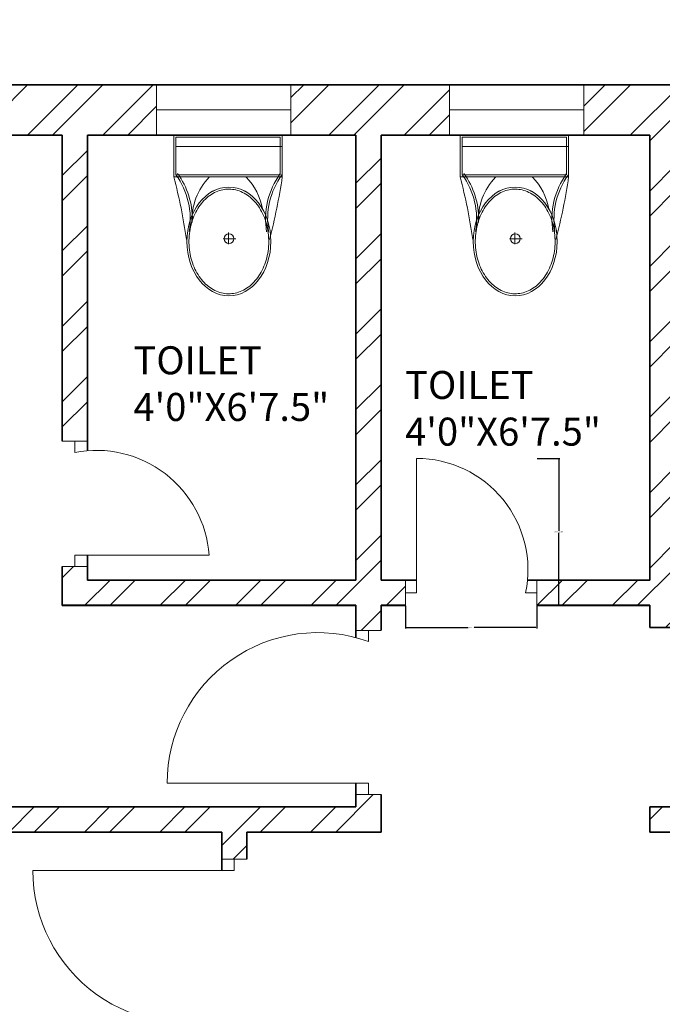
# Model space of a CAD drawing. Units: inches. Extents: x 2120 to 4013, y 1390 to 3019.
# Tile 33 of 59: x 2356 to 2470, y 2188 to 2364. Entities that reach past the tile are written whole.
import ezdxf

# ---------------------------------------------------------------- set-up
doc = ezdxf.new("R2010")
doc.units = ezdxf.units.IN
for name, color, linetype, lineweight in [('A-ANNO-DIMS', 2, 'Continuous', 18), ('A-AREA-IDEN', 7, 'Continuous', 18), ('A-DOOR', 3, 'Continuous', 18), ('A-FLOR-FIXT', 9, 'Continuous', 18), ('A-GLAZ', 4, 'Continuous', 18), ('A-WALL', 7, 'Continuous', 35), ('A-WALL-PATT', 252, 'Continuous', 13)]:
    doc.layers.add(name, color=color, linetype=linetype, lineweight=lineweight)
doc.styles.get("Standard").update_dxf_attribs({"font": 'arial.ttf'})
doc.dimstyles.get("Standard").update_dxf_attribs({"dimtxt": 0.18, "dimasz": 0.18, "dimexe": 0.18, "dimexo": 0.0625, "dimgap": 0.09, "dimtad": 0, "dimtih": 1, "dimtoh": 1, "dimdec": 4, "dimzin": 0, "dimdsep": 46, "dimtxsty": 'Standard', "dimcen": 0.09, "dimadec": 0, "dimazin": 0, "dimtfac": 1, "dimtdec": 4, "dimtofl": 0, "dimtmove": 0, "dimatfit": 3, "dimfxl": 1, "dimtolj": 1, "dimtzin": 0, "dimarcsym": 0})

# ---------------------------------------------------------------- blocks, each defined once
blk = doc.blocks.new('A$C31115884')
for p, q in [((257.5, 466.4), (257.5, 523.2)), ((283.1, 497.7), (223.4, 497.7)), ((0, 200), (0, 0)), ((520, 200), (0, 200)), ((10, 190), (10, 10)), ((510, 190), (10, 190)), ((510, 10), (510, 190)), ((520, 0), (520, 200)), ((510, 54.5), (0, 54.5)), ((10, 10), (510, 10)), ((0, 0), (520, 0))]:
    blk.add_line(p, q)
blk.add_circle((255.6, 496.4), 23.6)
for centre, radius, start, end in [((2777.7, -204.6), 2807, 165.4549, 171.7133), ((3237, 905), 2807, 188.2867, 194.5451), ((-294.5, 403.3), 364.7, 324.2091, 9.3499), ((-294.5, 403.3), 374.7, 324.2091, 9.3499), ((805.8, 403.3), 364.7, 170.6501, 215.7909), ((139.5, 406.2), 293.5, 315.8436, 2.6563), ((805.8, 403.3), 374.7, 179.2036, 215.7909), ((383.6, 406.2), 293.5, 190.2774, 224.1564)]:
    blk.add_arc(centre, radius, start, end)
blk.add_ellipse((256.2, 509.9), major_axis=(0, -260.7), ratio=0.772727)
blk.add_open_spline([(256.2, 259.2), (263.1, 259.2), (270, 259.7), (287.8, 262.3), (298.7, 265.1), (319.9, 273.1), (330.2, 278.4), (350.1, 291.1), (359.7, 298.7), (377.7, 315.9), (386.2, 325.5), (401.7, 346.6), (408.8, 358.1), (421.3, 382.5), (426.8, 395.5), (435.9, 422.4), (439.5, 436.4), (444.8, 465.1), (446.5, 479.7), (447.9, 509.2), (447.6, 524), (445, 553.3), (442.7, 567.8), (436.3, 596), (432.1, 609.7), (421.9, 636), (416, 648.6), (402.5, 672.1), (395, 683), (378.6, 703), (369.8, 712.1), (351.1, 728), (341.3, 734.8), (320.9, 746.2), (310.4, 750.7), (288.9, 757.3), (278, 759.4), (256, 761), (245, 760.6), (223.1, 757.2), (212.3, 754.3), (191.1, 746.1), (180.8, 740.7), (160.9, 727.8), (151.4, 720.1), (133.5, 702.7), (125.1, 693), (109.6, 671.7), (102.6, 660.2), (90.2, 635.7), (84.9, 622.7), (76, 595.6), (72.4, 581.6), (67.2, 552.9), (65.6, 538.2), (64.4, 508.8), (64.8, 494), (67.5, 464.7), (69.9, 450.2), (76.6, 422), (80.8, 408.3), (91.1, 382.2), (97.2, 369.7), (110.8, 346.3), (118.4, 335.4), (134.8, 315.6), (143.7, 306.7), (162.4, 290.9), (172.3, 284.2), (192.8, 273), (203.3, 268.6), (224.8, 262.2), (235.8, 260.2), (249.9, 259.3), (253, 259.2), (256.2, 259.2)], degree=3, knots=[0, 0, 0, 0, 0.110105, 0.110105, 0.285049, 0.285049, 0.459994, 0.459994, 0.634938, 0.634938, 0.809882, 0.809882, 0.984827, 0.984827, 1.159771, 1.159771, 1.334715, 1.334715, 1.50966, 1.50966, 1.684604, 1.684604, 1.859549, 1.859549, 2.034493, 2.034493, 2.209437, 2.209437, 2.384382, 2.384382, 2.559326, 2.559326, 2.73427, 2.73427, 2.909215, 2.909215, 3.084159, 3.084159, 3.259103, 3.259103, 3.434048, 3.434048, 3.608992, 3.608992, 3.783936, 3.783936, 3.958881, 3.958881, 4.133825, 4.133825, 4.30877, 4.30877, 4.483714, 4.483714, 4.658658, 4.658658, 4.833603, 4.833603, 5.008547, 5.008547, 5.183491, 5.183491, 5.358436, 5.358436, 5.53338, 5.53338, 5.708324, 5.708324, 5.883269, 5.883269, 6.058213, 6.058213, 6.233158, 6.233158, 6.283185, 6.283185, 6.283185, 6.283185])
blk = doc.blocks.new('DOOR-SWING-24IN-96p73DEG')
for p, q in [((4.5, 22.36), (0, 22.36)), ((0, 22.36), (2.25, 22.36)), ((2.25, 22.36), (2.25, 20.36)), ((2.25, 0), (2.25, 2)), ((2.25, 2), (26.25, 2)), ((4.5, 0), (0, 0)), ((0, 0), (2.25, 0))]:
    blk.add_line(p, q)
blk.add_arc((6.09, 0.51), 20.22, 4.2154, 100.9483)
blk = doc.blocks.new('DOOR-SWING-24IN-101p88DEG')
for p, q in [((2, 2.25), (2, 26.25)), ((0, 4.5), (0, 0)), ((23.48, 4.5), (23.48, 0)), ((0, 0), (0, 2.25)), ((0, 2.25), (2, 2.25)), ((23.48, 2.25), (21.48, 2.25)), ((23.48, 0), (23.48, 2.25))]:
    blk.add_line(p, q)
blk.add_arc((2, 6.35), 19.9, 348.1217, 90)
blk = doc.blocks.new('DOOR-SWING-36IN-109p78DEG')
for p, q in [((33.75, 29.31), (38.25, 29.31)), ((38.25, 29.31), (36, 29.31)), ((36, 29.31), (36, 27.31)), ((36, 2), (0, 2)), ((36, 0), (36, 2)), ((33.75, 0), (38.25, 0)), ((38.25, 0), (35.24, 0)), ((35.24, 0), (36, 0))]:
    blk.add_line(p, q)
blk.add_arc((26.9, 2), 26.9, 70.2228, 180)
blk = doc.blocks.new('DOOR-SWING-36IN-108p68DEG')
for p, q in [((38.25, 29.83), (33.75, 29.83)), ((33.75, 29.83), (36, 29.83)), ((36, 29.83), (36, 27.83)), ((36, 27.83), (0, 27.83)), ((36, 0), (36, 2)), ((33.75, 0), (38.25, 0)), ((38.25, 0), (36, 0))]:
    blk.add_line(p, q)
blk.add_arc((27.27, 27.83), 27.27, 180, 288.6764)
blk = doc.blocks.new('WIN-PLAN-24IN')
for p, q in [((0, 0), (0, 9)), ((0, 9), (0, 4.5)), ((24, 4.5), (24, 9)), ((24, 9), (24, 0)), ((0, 4.5), (24, 4.5)), ((0, 0), (0, 0))]:
    blk.add_line(p, q)
blk = doc.blocks.new('WIN-PLAN-24IN-02')
for p, q in [((0, 0), (0, 9)), ((0, 9), (0, 4.5)), ((24, 4.5), (24, 9)), ((24, 9), (24, 0)), ((0, 4.5), (24, 4.5))]:
    blk.add_line(p, q)
blk = doc.blocks.new('*D115')
at = {"layer": 'A-ANNO-DIMS', "color": 0, "lineweight": -2, "transparency": 16777216}
for p, q in [((2448.11, 2285.78), (2452.17, 2285.78)), ((2451.99, 2285.6), (2451.99, 2272.84)), ((2451.99, 2259.71), (2451.99, 2272.47)), ((2448.11, 2259.53), (2452.17, 2259.53))]:
    blk.add_line(p, q, dxfattribs=at)
at = {"layer": 'A-ANNO-DIMS', "color": 0, "transparency": 16777216}
for points in [[(2451.96, 2285.6), (2452.02, 2285.6), (2451.99, 2285.78)], [(2451.96, 2259.71), (2452.02, 2259.71), (2451.99, 2259.53)]]:
    blk.add_solid(points, dxfattribs=at)
at = {"layer": 'Defpoints', "color": 0, "transparency": 16777216}
for p in [(2448.05, 2285.78), (2451.99, 2285.78), (2448.05, 2259.53)]:
    blk.add_point(p, dxfattribs=at)
at = {"layer": 'A-ANNO-DIMS', "color": 0, "transparency": 16777216, "insert": (2451.99, 2272.66), "char_height": 0.18, "attachment_point": 5}
blk.add_mtext('\\A1;SWING 26 TYP.', dxfattribs=at)
blk = doc.blocks.new('*D116')
at = {"layer": 'A-ANNO-DIMS', "color": 0, "lineweight": -2, "transparency": 16777216}
for p, q in [((2424.57, 2259.47), (2424.57, 2255.41)), ((2448.05, 2259.47), (2448.05, 2255.41)), ((2424.75, 2255.59), (2435.78, 2255.59)), ((2447.87, 2255.59), (2436.84, 2255.59))]:
    blk.add_line(p, q, dxfattribs=at)
at = {"layer": 'A-ANNO-DIMS', "color": 0, "transparency": 16777216}
for points in [[(2424.75, 2255.62), (2424.75, 2255.56), (2424.57, 2255.59)], [(2447.87, 2255.62), (2447.87, 2255.56), (2448.05, 2255.59)]]:
    blk.add_solid(points, dxfattribs=at)
at = {"layer": 'Defpoints', "color": 0, "transparency": 16777216}
for p in [(2424.57, 2259.53), (2448.05, 2259.53), (2448.05, 2255.59)]:
    blk.add_point(p, dxfattribs=at)
at = {"layer": 'A-ANNO-DIMS', "color": 0, "transparency": 16777216, "insert": (2436.31, 2255.59), "char_height": 0.18, "attachment_point": 5}
blk.add_mtext('\\A1;23 TYP.', dxfattribs=at)
blk = doc.blocks.new('*D211')
at = {"layer": 'A-ANNO-DIMS', "color": 0, "lineweight": -2, "transparency": 16777216}
for p, q in [((2262.73, 2352.59), (2262.73, 2397.71)), ((2262.91, 2397.53), (2635.95, 2397.53)), ((3009.55, 2397.53), (2636.52, 2397.53)), ((3009.73, 2352.59), (3009.73, 2397.71))]:
    blk.add_line(p, q, dxfattribs=at)
at = {"layer": 'A-ANNO-DIMS', "color": 0, "transparency": 16777216}
for points in [[(2262.91, 2397.56), (2262.91, 2397.5), (2262.73, 2397.53)], [(3009.55, 2397.56), (3009.55, 2397.5), (3009.73, 2397.53)]]:
    blk.add_solid(points, dxfattribs=at)
at = {"layer": 'Defpoints', "color": 0, "transparency": 16777216}
for p in [(3009.73, 2397.53), (2262.73, 2352.53), (3009.73, 2352.53)]:
    blk.add_point(p, dxfattribs=at)
at = {"layer": 'A-ANNO-DIMS', "color": 0, "transparency": 16777216, "insert": (2636.23, 2397.53), "char_height": 0.18, "attachment_point": 5}
blk.add_mtext('\\A1;747', dxfattribs=at)

msp = doc.modelspace()

# ---------------------------------------------------------------- hatches: boundary and pattern name
at = {"layer": 'A-WALL-PATT'}
h = msp.add_hatch(dxfattribs=at)
h.set_pattern_fill('ANSI32', color=256)
h.paths.add_polyline_path([(2271.7331, 2343.531), (2283.3788, 2343.531), (2283.3788, 2348.031), (2283.3788, 2352.5306), (2262.7331, 2352.5306), (2262.7331, 2182.638), (2267.2331, 2182.638), (2271.7331, 2182.638), (2271.7331, 2219.031), (2391.7331, 2219.031), (2391.7331, 2214.189), (2393.9831, 2214.189), (2396.2331, 2214.189), (2396.2331, 2219.031), (2420.2331, 2219.031), (2420.2331, 2225.7535), (2417.2197, 2225.7535), (2415.7331, 2225.7535), (2415.7331, 2223.5306), (2271.7331, 2223.5306)])
h.paths.add_polyline_path([(2380.0942, 2352.5306), (2343.3788, 2352.5306), (2343.3788, 2343.531), (2363.2331, 2343.531), (2363.2331, 2288.8489), (2365.4831, 2288.8489), (2367.7331, 2288.8489), (2367.7331, 2343.531), (2380.0942, 2343.531)], flags=17)
h.paths.add_polyline_path([(2432.4339, 2352.5306), (2404.0943, 2352.5306), (2404.0943, 2343.531), (2415.7331, 2343.531), (2415.7331, 2264.0306), (2367.7331, 2264.0306), (2367.7331, 2266.4872), (2363.2331, 2266.4872), (2363.2331, 2259.531), (2367.7331, 2259.531), (2415.7331, 2259.531), (2415.7331, 2255.0658), (2420.2331, 2255.0658), (2420.2331, 2259.531), (2424.5717, 2259.531), (2424.5717, 2261.781), (2424.5717, 2264.0306), (2420.2331, 2264.0306), (2420.2331, 2343.531), (2432.4339, 2343.531)])
h.paths.add_polyline_path([(2508.9115, 2352.5306), (2456.4339, 2352.5306), (2456.4339, 2343.531), (2468.2331, 2343.531), (2468.2331, 2264.0306), (2448.0487, 2264.0306), (2448.0487, 2259.531), (2468.2331, 2259.531), (2468.2331, 2255.5496), (2472.7331, 2255.5496), (2472.7331, 2343.531), (2508.9115, 2343.531)])
h.paths.add_polyline_path([(2637.7331, 2352.5306), (2544.9116, 2352.5306), (2544.9116, 2343.531), (2589.7331, 2343.531), (2633.2331, 2343.531), (2637.7331, 2343.531)])
h.paths.add_polyline_path([(2594.2331, 2343.5306), (2589.7331, 2343.5306), (2589.7331, 2259.5306), (2589.7331, 2252.4915), (2591.9831, 2252.4915), (2594.2331, 2252.4915)])
h.paths.add_polyline_path([(2637.7331, 2223.5306), (2594.2331, 2223.5306), (2594.2331, 2230.1988), (2591.9831, 2230.1988), (2589.7331, 2230.1988), (2589.7331, 2223.5306), (2472.7331, 2223.5306), (2468.2331, 2223.5306), (2468.2331, 2219.031), (2628.7331, 2219.031), (2628.7331, 2138.031), (2637.7331, 2138.031)])
h.paths.add_polyline_path([(3822.6535, 2458.4402), (3874.9468, 2458.4402), (3874.9468, 2476.9866), (3822.6535, 2476.9866)], flags=9)
h.paths.add_polyline_path([(3834.6921, 2781.8174), (3935.9206, 2781.8174), (3935.9206, 2800.3638), (3834.6921, 2800.3638)], flags=9)
h.paths.add_polyline_path([(3832.2843, 2837.9683), (3884.5776, 2837.9683), (3884.5776, 2856.5146), (3832.2843, 2856.5146)], flags=9)
h.paths.add_polyline_path([(3830.9388, 2861.4782), (3956.8958, 2861.4782), (3956.8958, 2880.0245), (3830.9388, 2880.0245)], flags=9)
h.paths.add_polyline_path([(3870.6966, 2352.5752), (3887.9272, 2352.5752), (3887.9272, 2377.3037), (3870.6966, 2377.3037)], flags=9)
h.paths.add_polyline_path([(3289.2701, 2413.161), (3435.2223, 2413.161), (3435.2223, 2450.2538), (3289.2701, 2450.2538)], flags=9)
h.paths.add_polyline_path([(2487.6944, 2414.3601), (2637.8335, 2414.3601), (2637.8335, 2451.4528), (2487.6944, 2451.4528)], flags=9)
h.paths.add_polyline_path([(2567.3724, 1457.9199), (2815.296, 1457.9199), (2815.296, 1495.0127), (2567.3724, 1495.0127)], flags=9)
h.paths.add_polyline_path([(2655.3825, 2093.2363), (2685.9555, 2093.2363), (2685.9555, 2111.8937), (2655.3825, 2111.8937)], flags=9)
h.paths.add_polyline_path([(2543.9218, 1550.6671), (2587.8406, 1550.6671), (2587.8406, 1569.3244), (2543.9218, 1569.3244)], flags=9)
h.paths.add_polyline_path([(2905.1384, 1543.8113), (2949.0572, 1543.8113), (2949.0572, 1562.4686), (2905.1384, 1562.4686)], flags=9)
h.paths.add_polyline_path([(2736.4118, 1702.4736), (2784.2153, 1702.4736), (2784.2153, 1721.1309), (2736.4118, 1721.1309)], flags=9)
h.paths.add_polyline_path([(2912.8666, 1710.4168), (2951.707, 1710.4168), (2951.707, 1729.0741), (2912.8666, 1729.0741)], flags=9)
h.paths.add_polyline_path([(2923.5785, 1763.5038), (2959.7279, 1763.5038), (2959.7279, 1782.1611), (2923.5785, 1782.1611)], flags=9)
h.paths.add_polyline_path([(2925.2114, 1809.6137), (2967.1861, 1809.6137), (2967.1861, 1828.271), (2925.2114, 1828.271)], flags=9)
h.paths.add_polyline_path([(2996.2711, 1878.9003), (2996.2711, 1913.109), (2977.6138, 1913.109), (2977.6138, 1878.9003)], flags=9)
h.paths.add_polyline_path([(2883.0859, 1895.7192), (2927.1855, 1895.7192), (2927.1855, 1914.3766), (2883.0859, 1914.3766)], flags=9)
h.paths.add_polyline_path([(2787.3924, 1810.8013), (2841.0213, 1810.8013), (2841.0213, 1829.4587), (2787.3924, 1829.4587)], flags=9)
h.paths.add_polyline_path([(2775.6399, 2101.7395), (2829.2689, 2101.7395), (2829.2689, 2120.3968), (2775.6399, 2120.3968)], flags=9)
h.paths.add_polyline_path([(2913.0263, 2075.817), (2951.8667, 2075.817), (2951.8667, 2094.4744), (2913.0263, 2094.4744)], flags=9)
h.paths.add_polyline_path([(2929.966, 2133.3669), (2966.1154, 2133.3669), (2966.1154, 2152.0243), (2929.966, 2152.0243)], flags=9)
h.paths.add_polyline_path([(2932.7502, 2182.6088), (2968.8996, 2182.6088), (2968.8996, 2201.2662), (2932.7502, 2201.2662)], flags=9)
h.paths.add_polyline_path([(2996.0681, 2266.3173), (2996.0681, 2300.5261), (2977.4108, 2300.5261), (2977.4108, 2266.3173)], flags=9)
h.paths.add_polyline_path([(2885.1039, 2279.2186), (2929.2035, 2279.2186), (2929.2035, 2297.8759), (2885.1039, 2297.8759)], flags=9)
h.paths.add_polyline_path([(2735.7042, 2218.3197), (2783.5078, 2218.3197), (2783.5078, 2236.9771), (2735.7042, 2236.9771)], flags=9)
h.paths.add_polyline_path([(2635.6049, 2044.0085), (2648.9678, 2044.0085), (2648.9678, 2054.312), (2635.6049, 2054.312)], flags=9)
h.paths.add_polyline_path([(2714.0148, 1923.0473), (2727.3777, 1923.0473), (2727.3777, 1933.3508), (2714.0148, 1933.3508)], flags=9)
h.paths.add_polyline_path([(2709.0345, 1988.1628), (2722.3974, 1988.1628), (2722.3974, 1998.4663), (2709.0345, 1998.4663)], flags=9)
h.paths.add_polyline_path([(2592.8935, 1962.1763), (2606.2564, 1962.1763), (2606.2564, 1972.4799), (2592.8935, 1972.4799)], flags=9)
h.paths.add_polyline_path([(2618.3996, 1985.9724), (2644.1942, 1985.9724), (2644.1942, 1996.2759), (2618.3996, 1996.2759)], flags=9)
h.paths.add_polyline_path([(2601.279, 1920.5869), (2614.6419, 1920.5869), (2614.6419, 1930.8904), (2601.279, 1930.8904)], flags=9)
h.paths.add_polyline_path([(2692.3278, 1932.7645), (2704.5311, 1932.7645), (2704.5311, 1943.0681), (2692.3278, 1943.0681)], flags=9)
h.paths.add_polyline_path([(2311.122, 1672.7318), (2355.0408, 1672.7318), (2355.0408, 1691.3892), (2311.122, 1691.3892)], flags=9)
h.paths.add_polyline_path([(2456.2551, 1632.3198), (2492.4796, 1632.3198), (2492.4796, 1650.9772), (2456.2551, 1650.9772)], flags=9)
h.paths.add_polyline_path([(2401.0766, 1631.4793), (2437.301, 1631.4793), (2437.301, 1650.1367), (2401.0766, 1650.1367)], flags=9)
h.paths.add_polyline_path([(2546.7054, 1700.9235), (2594.509, 1700.9235), (2594.509, 1719.5809), (2546.7054, 1719.5809)], flags=9)
h.paths.add_polyline_path([(2445.4866, 1766.9937), (2497.5261, 1766.9937), (2497.5261, 1785.651), (2445.4866, 1785.651)], flags=9)
h.paths.add_polyline_path([(2287.9992, 1739.7675), (2326.8396, 1739.7675), (2326.8396, 1758.4248), (2287.9992, 1758.4248)], flags=9)
h.paths.add_polyline_path([(2458.5279, 1924.7607), (2510.5675, 1924.7607), (2510.5675, 1943.4181), (2458.5279, 1943.4181)], flags=9)
h.paths.add_polyline_path([(2309.2811, 1902.7642), (2345.4305, 1902.7642), (2345.4305, 1921.4215), (2309.2811, 1921.4215)], flags=9)
h.paths.add_polyline_path([(2490.7554, 2018.9392), (2530.7896, 2018.9392), (2530.7896, 2037.5965), (2490.7554, 2037.5965)], flags=9)
h.paths.add_polyline_path([(2402.143, 2024.7393), (2438.5414, 2024.7393), (2438.5414, 2043.3966), (2402.143, 2043.3966)], flags=9)
h.paths.add_polyline_path([(2287.856, 1931.7926), (2326.6964, 1931.7926), (2326.6964, 1950.4499), (2287.856, 1950.4499)], flags=9)
h.paths.add_polyline_path([(2281.7979, 2193.5771), (2320.6383, 2193.5771), (2320.6383, 2212.2344), (2281.7979, 2212.2344)], flags=25)
h.paths.add_polyline_path([(2484.0754, 2093.892), (2536.115, 2093.892), (2536.115, 2112.5494), (2484.0754, 2112.5494)], flags=9)
h.paths.add_polyline_path([(2624.7948, 2281.8639), (2624.7948, 2311.4137), (2606.1375, 2311.4137), (2606.1375, 2281.8639)], flags=9)
h.paths.add_polyline_path([(2507.5036, 2290.3639), (2541.934, 2290.3639), (2541.934, 2309.0212), (2507.5036, 2309.0212)], flags=9)
h.paths.add_polyline_path([(2423.1076, 2285.2202), (2459.332, 2285.2202), (2459.332, 2303.8776), (2423.1076, 2303.8776)], flags=9)
h.paths.add_polyline_path([(2374.5467, 2289.6272), (2410.7711, 2289.6272), (2410.7711, 2308.2846), (2374.5467, 2308.2846)], flags=25)
h.paths.add_polyline_path([(2277.4907, 2227.5651), (2316.3311, 2227.5651), (2316.3311, 2246.2224), (2277.4907, 2246.2224)], flags=25)
h.paths.add_polyline_path([(2655.3825, 2093.2367), (2685.9555, 2093.2367), (2685.9555, 2111.894), (2655.3825, 2111.894)], flags=9)
h.paths.add_polyline_path([(2543.9217, 1550.6674), (2587.8406, 1550.6674), (2587.8406, 1569.3247), (2543.9217, 1569.3247)], flags=9)
h.paths.add_polyline_path([(2905.1384, 1543.8116), (2949.0572, 1543.8116), (2949.0572, 1562.4689), (2905.1384, 1562.4689)], flags=9)
h.paths.add_polyline_path([(2736.4118, 1702.4739), (2784.2153, 1702.4739), (2784.2153, 1721.1312), (2736.4118, 1721.1312)], flags=9)
h.paths.add_polyline_path([(2912.8666, 1710.4171), (2951.707, 1710.4171), (2951.707, 1729.0744), (2912.8666, 1729.0744)], flags=9)
h.paths.add_polyline_path([(2923.5785, 1763.5041), (2959.7279, 1763.5041), (2959.7279, 1782.1614), (2923.5785, 1782.1614)], flags=9)
h.paths.add_polyline_path([(2925.2114, 1809.614), (2967.1861, 1809.614), (2967.1861, 1828.2713), (2925.2114, 1828.2713)], flags=9)
h.paths.add_polyline_path([(2996.2711, 1878.9006), (2996.2711, 1913.1094), (2977.6137, 1913.1094), (2977.6137, 1878.9006)], flags=9)
h.paths.add_polyline_path([(2883.0859, 1895.7195), (2927.1855, 1895.7195), (2927.1855, 1914.3769), (2883.0859, 1914.3769)], flags=9)
h.paths.add_polyline_path([(2787.3924, 1810.8016), (2841.0213, 1810.8016), (2841.0213, 1829.459), (2787.3924, 1829.459)], flags=9)
h.paths.add_polyline_path([(2775.6399, 2101.7398), (2829.2688, 2101.7398), (2829.2688, 2120.3971), (2775.6399, 2120.3971)], flags=9)
h.paths.add_polyline_path([(2913.0263, 2075.8173), (2951.8667, 2075.8173), (2951.8667, 2094.4747), (2913.0263, 2094.4747)], flags=9)
h.paths.add_polyline_path([(2929.966, 2133.3672), (2966.1154, 2133.3672), (2966.1154, 2152.0246), (2929.966, 2152.0246)], flags=9)
h.paths.add_polyline_path([(2932.7502, 2182.6091), (2968.8996, 2182.6091), (2968.8996, 2201.2665), (2932.7502, 2201.2665)], flags=9)
h.paths.add_polyline_path([(2996.0681, 2266.3176), (2996.0681, 2300.5264), (2977.4108, 2300.5264), (2977.4108, 2266.3176)], flags=9)
h.paths.add_polyline_path([(2885.1039, 2279.2189), (2929.2035, 2279.2189), (2929.2035, 2297.8762), (2885.1039, 2297.8762)], flags=9)
h.paths.add_polyline_path([(2735.7042, 2218.32), (2783.5078, 2218.32), (2783.5078, 2236.9774), (2735.7042, 2236.9774)], flags=9)
h.paths.add_polyline_path([(2635.6048, 2044.0088), (2648.9677, 2044.0088), (2648.9677, 2054.3123), (2635.6048, 2054.3123)], flags=9)
h.paths.add_polyline_path([(2714.0148, 1923.0476), (2727.3777, 1923.0476), (2727.3777, 1933.3511), (2714.0148, 1933.3511)], flags=9)
h.paths.add_polyline_path([(2709.0345, 1988.1631), (2722.3974, 1988.1631), (2722.3974, 1998.4666), (2709.0345, 1998.4666)], flags=9)
h.paths.add_polyline_path([(2592.8935, 1962.1766), (2606.2564, 1962.1766), (2606.2564, 1972.4802), (2592.8935, 1972.4802)], flags=9)
h.paths.add_polyline_path([(2618.3995, 1985.9727), (2644.1942, 1985.9727), (2644.1942, 1996.2762), (2618.3995, 1996.2762)], flags=9)
h.paths.add_polyline_path([(2601.279, 1920.5872), (2614.6419, 1920.5872), (2614.6419, 1930.8908), (2601.279, 1930.8908)], flags=9)
h.paths.add_polyline_path([(2692.3278, 1932.7648), (2704.5311, 1932.7648), (2704.5311, 1943.0684), (2692.3278, 1943.0684)], flags=9)
h.paths.add_polyline_path([(2311.122, 1672.7321), (2355.0408, 1672.7321), (2355.0408, 1691.3895), (2311.122, 1691.3895)], flags=9)
h.paths.add_polyline_path([(2456.2551, 1632.3201), (2492.4795, 1632.3201), (2492.4795, 1650.9775), (2456.2551, 1650.9775)], flags=9)
h.paths.add_polyline_path([(2401.0766, 1631.4796), (2437.301, 1631.4796), (2437.301, 1650.137), (2401.0766, 1650.137)], flags=9)
h.paths.add_polyline_path([(2546.7054, 1700.9238), (2594.509, 1700.9238), (2594.509, 1719.5812), (2546.7054, 1719.5812)], flags=9)
h.paths.add_polyline_path([(2445.4866, 1766.994), (2497.5261, 1766.994), (2497.5261, 1785.6513), (2445.4866, 1785.6513)], flags=9)
h.paths.add_polyline_path([(2287.9992, 1739.7678), (2326.8396, 1739.7678), (2326.8396, 1758.4251), (2287.9992, 1758.4251)], flags=9)
h.paths.add_polyline_path([(2458.5279, 1924.7611), (2510.5675, 1924.7611), (2510.5675, 1943.4184), (2458.5279, 1943.4184)], flags=9)
h.paths.add_polyline_path([(2309.2811, 1902.7645), (2345.4305, 1902.7645), (2345.4305, 1921.4218), (2309.2811, 1921.4218)], flags=9)
h.paths.add_polyline_path([(2490.7554, 2018.9395), (2530.7895, 2018.9395), (2530.7895, 2037.5968), (2490.7554, 2037.5968)], flags=9)
h.paths.add_polyline_path([(2402.143, 2024.7396), (2438.5413, 2024.7396), (2438.5413, 2043.3969), (2402.143, 2043.3969)], flags=9)
h.paths.add_polyline_path([(2287.856, 1931.7929), (2326.6964, 1931.7929), (2326.6964, 1950.4502), (2287.856, 1950.4502)], flags=9)
h.paths.add_polyline_path([(2281.7979, 2193.5774), (2320.6383, 2193.5774), (2320.6383, 2212.2347), (2281.7979, 2212.2347)], flags=25)
h.paths.add_polyline_path([(2484.0754, 2093.8924), (2536.115, 2093.8924), (2536.115, 2112.5497), (2484.0754, 2112.5497)], flags=9)
h.paths.add_polyline_path([(2624.7948, 2281.8642), (2624.7948, 2311.414), (2606.1374, 2311.414), (2606.1374, 2281.8642)], flags=9)
h.paths.add_polyline_path([(2507.5035, 2290.3642), (2541.934, 2290.3642), (2541.934, 2309.0215), (2507.5035, 2309.0215)], flags=9)
h.paths.add_polyline_path([(2423.1075, 2285.2205), (2459.332, 2285.2205), (2459.332, 2303.8779), (2423.1075, 2303.8779)], flags=9)
h.paths.add_polyline_path([(2374.5467, 2289.6275), (2410.7711, 2289.6275), (2410.7711, 2308.2849), (2374.5467, 2308.2849)], flags=25)
h.paths.add_polyline_path([(2277.4907, 2227.5654), (2316.3311, 2227.5654), (2316.3311, 2246.2227), (2277.4907, 2246.2227)], flags=25)
h = msp.add_hatch(dxfattribs=at)
h.set_pattern_fill('ANSI32', color=256)
h.paths.add_polyline_path([(2271.7331, 1980.389), (2262.7331, 1980.389), (2262.7331, 1912.8434), (2267.2331, 1912.8434), (2271.7331, 1912.8434), (2271.7331, 1922.531), (2351.2331, 1922.531), (2351.2331, 1901.4728), (2355.7331, 1901.4728), (2355.7331, 1922.531), (2357.9815, 1922.531), (2357.9815, 1926.5306), (2271.7331, 1926.5306)])
h.paths.add_polyline_path([(2589.2331, 1949.1622), (2584.7331, 1949.1622), (2580.2331, 1949.1622), (2580.2331, 1874.5306), (2355.7331, 1874.5306), (2355.7331, 1880.1922), (2351.2331, 1880.1922), (2351.2331, 1874.5306), (2271.7331, 1874.5306), (2271.7331, 1888.8431), (2262.7331, 1888.8431), (2262.7331, 1842.2909), (2267.2331, 1842.2909), (2271.7331, 1842.2909), (2271.7331, 1865.531), (2415.7331, 1865.531), (2415.7331, 1779.7286), (2420.2331, 1779.7286), (2420.2331, 1865.531), (2589.2331, 1865.531)])
h.paths.add_polyline_path([(2271.7331, 1782.2906), (2262.7331, 1782.2906), (2262.7331, 1711.4639), (2267.2331, 1711.4639), (2271.7331, 1711.4639), (2271.7331, 1738.031), (2420.2331, 1738.031), (2420.2331, 1742.531), (2420.2331, 1747.3376), (2417.9831, 1747.3376), (2415.7331, 1747.3376), (2415.7331, 1742.5306), (2271.7331, 1742.5306)])
h.paths.add_polyline_path([(2271.7331, 1627.031), (2362.3957, 1627.031), (2362.3957, 1629.281), (2362.3957, 1631.5306), (2271.7331, 1631.5306), (2271.7331, 1675.4636), (2262.7331, 1675.4636), (2262.7331, 1581.531), (2405.3032, 1581.531), (2405.3032, 1586.031), (2405.3032, 1590.5306), (2396.2331, 1590.5306), (2396.2331, 1691.4513), (2418.7206, 1691.4513), (2418.7206, 1695.951), (2396.2331, 1695.951), (2391.7331, 1695.951), (2391.7331, 1631.5306), (2386.7425, 1631.5306), (2386.7425, 1629.2806), (2386.7425, 1627.031), (2391.7331, 1627.031), (2391.7331, 1586.1709), (2271.7331, 1586.1709)])
h.paths.add_polyline_path([(2459.6703, 1590.5306), (2429.3032, 1590.5306), (2429.3032, 1581.531), (2459.6703, 1581.531), (2459.6703, 1586.031)])
h.paths.add_polyline_path([(2501.2331, 1590.531), (2501.2331, 1665.0195), (2498.9831, 1665.0195), (2496.7331, 1665.0195), (2496.7331, 1590.5306), (2483.8201, 1590.5306), (2483.8201, 1590.1579), (2483.6704, 1590.1579), (2483.6704, 1581.531), (2505.0196, 1581.531), (2505.0196, 1583.781), (2505.0196, 1586.0306), (2501.2331, 1586.0306)])
h.paths.add_polyline_path([(2544.1361, 1583.781), (2544.1361, 1586.0306), (2527.1368, 1586.0306), (2527.1368, 1583.7806), (2527.1368, 1581.531), (2544.1361, 1581.531)])
h.paths.add_polyline_path([(3822.6535, 2458.4402), (3874.9468, 2458.4402), (3874.9468, 2476.9866), (3822.6535, 2476.9866)], flags=9)
h.paths.add_polyline_path([(3834.6921, 2781.8174), (3935.9206, 2781.8174), (3935.9206, 2800.3638), (3834.6921, 2800.3638)], flags=9)
h.paths.add_polyline_path([(3832.2843, 2837.9683), (3884.5776, 2837.9683), (3884.5776, 2856.5146), (3832.2843, 2856.5146)], flags=9)
h.paths.add_polyline_path([(3830.9388, 2861.4782), (3956.8958, 2861.4782), (3956.8958, 2880.0245), (3830.9388, 2880.0245)], flags=9)
h.paths.add_polyline_path([(3870.6966, 2352.5752), (3887.9272, 2352.5752), (3887.9272, 2377.3037), (3870.6966, 2377.3037)], flags=9)
h.paths.add_polyline_path([(3289.2701, 2413.161), (3435.2223, 2413.161), (3435.2223, 2450.2538), (3289.2701, 2450.2538)], flags=9)
h.paths.add_polyline_path([(2487.6944, 2414.3601), (2637.8335, 2414.3601), (2637.8335, 2451.4528), (2487.6944, 2451.4528)], flags=9)
h.paths.add_polyline_path([(2567.3724, 1457.9199), (2815.296, 1457.9199), (2815.296, 1495.0127), (2567.3724, 1495.0127)], flags=9)
h.paths.add_polyline_path([(2655.3825, 2093.2363), (2685.9555, 2093.2363), (2685.9555, 2111.8937), (2655.3825, 2111.8937)], flags=9)
h.paths.add_polyline_path([(2543.9218, 1550.6671), (2587.8406, 1550.6671), (2587.8406, 1569.3244), (2543.9218, 1569.3244)], flags=9)
h.paths.add_polyline_path([(2905.1384, 1543.8113), (2949.0572, 1543.8113), (2949.0572, 1562.4686), (2905.1384, 1562.4686)], flags=9)
h.paths.add_polyline_path([(2736.4118, 1702.4736), (2784.2153, 1702.4736), (2784.2153, 1721.1309), (2736.4118, 1721.1309)], flags=9)
h.paths.add_polyline_path([(2912.8666, 1710.4168), (2951.707, 1710.4168), (2951.707, 1729.0741), (2912.8666, 1729.0741)], flags=9)
h.paths.add_polyline_path([(2923.5785, 1763.5038), (2959.7279, 1763.5038), (2959.7279, 1782.1611), (2923.5785, 1782.1611)], flags=9)
h.paths.add_polyline_path([(2925.2114, 1809.6137), (2967.1861, 1809.6137), (2967.1861, 1828.271), (2925.2114, 1828.271)], flags=9)
h.paths.add_polyline_path([(2996.2711, 1878.9003), (2996.2711, 1913.109), (2977.6138, 1913.109), (2977.6138, 1878.9003)], flags=9)
h.paths.add_polyline_path([(2883.0859, 1895.7192), (2927.1855, 1895.7192), (2927.1855, 1914.3766), (2883.0859, 1914.3766)], flags=9)
h.paths.add_polyline_path([(2787.3924, 1810.8013), (2841.0213, 1810.8013), (2841.0213, 1829.4587), (2787.3924, 1829.4587)], flags=9)
h.paths.add_polyline_path([(2775.6399, 2101.7395), (2829.2689, 2101.7395), (2829.2689, 2120.3968), (2775.6399, 2120.3968)], flags=9)
h.paths.add_polyline_path([(2913.0263, 2075.817), (2951.8667, 2075.817), (2951.8667, 2094.4744), (2913.0263, 2094.4744)], flags=9)
h.paths.add_polyline_path([(2929.966, 2133.3669), (2966.1154, 2133.3669), (2966.1154, 2152.0243), (2929.966, 2152.0243)], flags=9)
h.paths.add_polyline_path([(2932.7502, 2182.6088), (2968.8996, 2182.6088), (2968.8996, 2201.2662), (2932.7502, 2201.2662)], flags=9)
h.paths.add_polyline_path([(2996.0681, 2266.3173), (2996.0681, 2300.5261), (2977.4108, 2300.5261), (2977.4108, 2266.3173)], flags=9)
h.paths.add_polyline_path([(2885.1039, 2279.2186), (2929.2035, 2279.2186), (2929.2035, 2297.8759), (2885.1039, 2297.8759)], flags=9)
h.paths.add_polyline_path([(2735.7042, 2218.3197), (2783.5078, 2218.3197), (2783.5078, 2236.9771), (2735.7042, 2236.9771)], flags=9)
h.paths.add_polyline_path([(2635.6049, 2044.0085), (2648.9678, 2044.0085), (2648.9678, 2054.312), (2635.6049, 2054.312)], flags=9)
h.paths.add_polyline_path([(2714.0148, 1923.0473), (2727.3777, 1923.0473), (2727.3777, 1933.3508), (2714.0148, 1933.3508)], flags=9)
h.paths.add_polyline_path([(2709.0345, 1988.1628), (2722.3974, 1988.1628), (2722.3974, 1998.4663), (2709.0345, 1998.4663)], flags=9)
h.paths.add_polyline_path([(2592.8935, 1962.1763), (2606.2564, 1962.1763), (2606.2564, 1972.4799), (2592.8935, 1972.4799)], flags=9)
h.paths.add_polyline_path([(2618.3996, 1985.9724), (2644.1942, 1985.9724), (2644.1942, 1996.2759), (2618.3996, 1996.2759)], flags=9)
h.paths.add_polyline_path([(2601.279, 1920.5869), (2614.6419, 1920.5869), (2614.6419, 1930.8904), (2601.279, 1930.8904)], flags=9)
h.paths.add_polyline_path([(2692.3278, 1932.7645), (2704.5311, 1932.7645), (2704.5311, 1943.0681), (2692.3278, 1943.0681)], flags=9)
h.paths.add_polyline_path([(2311.122, 1672.7318), (2355.0408, 1672.7318), (2355.0408, 1691.3892), (2311.122, 1691.3892)], flags=25)
h.paths.add_polyline_path([(2456.2551, 1632.3198), (2492.4796, 1632.3198), (2492.4796, 1650.9772), (2456.2551, 1650.9772)], flags=9)
h.paths.add_polyline_path([(2401.0766, 1631.4793), (2437.301, 1631.4793), (2437.301, 1650.1367), (2401.0766, 1650.1367)], flags=9)
h.paths.add_polyline_path([(2546.7054, 1700.9235), (2594.509, 1700.9235), (2594.509, 1719.5809), (2546.7054, 1719.5809)], flags=9)
h.paths.add_polyline_path([(2445.4866, 1766.9937), (2497.5261, 1766.9937), (2497.5261, 1785.651), (2445.4866, 1785.651)], flags=9)
h.paths.add_polyline_path([(2287.9992, 1739.7675), (2326.8396, 1739.7675), (2326.8396, 1758.4248), (2287.9992, 1758.4248)], flags=24)
h.paths.add_polyline_path([(2458.5279, 1924.7607), (2510.5675, 1924.7607), (2510.5675, 1943.4181), (2458.5279, 1943.4181)], flags=25)
h.paths.add_polyline_path([(2309.2811, 1902.7642), (2345.4305, 1902.7642), (2345.4305, 1921.4215), (2309.2811, 1921.4215)], flags=25)
h.paths.add_polyline_path([(2490.7554, 2018.9392), (2530.7896, 2018.9392), (2530.7896, 2037.5965), (2490.7554, 2037.5965)], flags=9)
h.paths.add_polyline_path([(2402.143, 2024.7393), (2438.5414, 2024.7393), (2438.5414, 2043.3966), (2402.143, 2043.3966)], flags=9)
h.paths.add_polyline_path([(2287.856, 1931.7926), (2326.6964, 1931.7926), (2326.6964, 1950.4499), (2287.856, 1950.4499)], flags=25)
h.paths.add_polyline_path([(2281.7979, 2193.5771), (2320.6383, 2193.5771), (2320.6383, 2212.2344), (2281.7979, 2212.2344)], flags=9)
h.paths.add_polyline_path([(2484.0754, 2093.892), (2536.115, 2093.892), (2536.115, 2112.5494), (2484.0754, 2112.5494)], flags=9)
h.paths.add_polyline_path([(2624.7948, 2281.8639), (2624.7948, 2311.4137), (2606.1375, 2311.4137), (2606.1375, 2281.8639)], flags=9)
h.paths.add_polyline_path([(2507.5036, 2290.3639), (2541.934, 2290.3639), (2541.934, 2309.0212), (2507.5036, 2309.0212)], flags=9)
h.paths.add_polyline_path([(2423.1076, 2285.2202), (2459.332, 2285.2202), (2459.332, 2303.8776), (2423.1076, 2303.8776)], flags=9)
h.paths.add_polyline_path([(2374.5467, 2289.6272), (2410.7711, 2289.6272), (2410.7711, 2308.2846), (2374.5467, 2308.2846)], flags=9)
h.paths.add_polyline_path([(2277.4907, 2227.5651), (2316.3311, 2227.5651), (2316.3311, 2246.2224), (2277.4907, 2246.2224)], flags=9)
h.paths.add_polyline_path([(2655.3825, 2093.2367), (2685.9555, 2093.2367), (2685.9555, 2111.894), (2655.3825, 2111.894)], flags=9)
h.paths.add_polyline_path([(2543.9217, 1550.6674), (2587.8406, 1550.6674), (2587.8406, 1569.3247), (2543.9217, 1569.3247)], flags=9)
h.paths.add_polyline_path([(2905.1384, 1543.8116), (2949.0572, 1543.8116), (2949.0572, 1562.4689), (2905.1384, 1562.4689)], flags=9)
h.paths.add_polyline_path([(2736.4118, 1702.4739), (2784.2153, 1702.4739), (2784.2153, 1721.1312), (2736.4118, 1721.1312)], flags=9)
h.paths.add_polyline_path([(2912.8666, 1710.4171), (2951.707, 1710.4171), (2951.707, 1729.0744), (2912.8666, 1729.0744)], flags=9)
h.paths.add_polyline_path([(2923.5785, 1763.5041), (2959.7279, 1763.5041), (2959.7279, 1782.1614), (2923.5785, 1782.1614)], flags=9)
h.paths.add_polyline_path([(2925.2114, 1809.614), (2967.1861, 1809.614), (2967.1861, 1828.2713), (2925.2114, 1828.2713)], flags=9)
h.paths.add_polyline_path([(2996.2711, 1878.9006), (2996.2711, 1913.1094), (2977.6137, 1913.1094), (2977.6137, 1878.9006)], flags=9)
h.paths.add_polyline_path([(2883.0859, 1895.7195), (2927.1855, 1895.7195), (2927.1855, 1914.3769), (2883.0859, 1914.3769)], flags=9)
h.paths.add_polyline_path([(2787.3924, 1810.8016), (2841.0213, 1810.8016), (2841.0213, 1829.459), (2787.3924, 1829.459)], flags=9)
h.paths.add_polyline_path([(2775.6399, 2101.7398), (2829.2688, 2101.7398), (2829.2688, 2120.3971), (2775.6399, 2120.3971)], flags=9)
h.paths.add_polyline_path([(2913.0263, 2075.8173), (2951.8667, 2075.8173), (2951.8667, 2094.4747), (2913.0263, 2094.4747)], flags=9)
h.paths.add_polyline_path([(2929.966, 2133.3672), (2966.1154, 2133.3672), (2966.1154, 2152.0246), (2929.966, 2152.0246)], flags=9)
h.paths.add_polyline_path([(2932.7502, 2182.6091), (2968.8996, 2182.6091), (2968.8996, 2201.2665), (2932.7502, 2201.2665)], flags=9)
h.paths.add_polyline_path([(2996.0681, 2266.3176), (2996.0681, 2300.5264), (2977.4108, 2300.5264), (2977.4108, 2266.3176)], flags=9)
h.paths.add_polyline_path([(2885.1039, 2279.2189), (2929.2035, 2279.2189), (2929.2035, 2297.8762), (2885.1039, 2297.8762)], flags=9)
h.paths.add_polyline_path([(2735.7042, 2218.32), (2783.5078, 2218.32), (2783.5078, 2236.9774), (2735.7042, 2236.9774)], flags=9)
h.paths.add_polyline_path([(2635.6048, 2044.0088), (2648.9677, 2044.0088), (2648.9677, 2054.3123), (2635.6048, 2054.3123)], flags=9)
h.paths.add_polyline_path([(2714.0148, 1923.0476), (2727.3777, 1923.0476), (2727.3777, 1933.3511), (2714.0148, 1933.3511)], flags=9)
h.paths.add_polyline_path([(2709.0345, 1988.1631), (2722.3974, 1988.1631), (2722.3974, 1998.4666), (2709.0345, 1998.4666)], flags=9)
h.paths.add_polyline_path([(2592.8935, 1962.1766), (2606.2564, 1962.1766), (2606.2564, 1972.4802), (2592.8935, 1972.4802)], flags=9)
h.paths.add_polyline_path([(2618.3995, 1985.9727), (2644.1942, 1985.9727), (2644.1942, 1996.2762), (2618.3995, 1996.2762)], flags=9)
h.paths.add_polyline_path([(2601.279, 1920.5872), (2614.6419, 1920.5872), (2614.6419, 1930.8908), (2601.279, 1930.8908)], flags=9)
h.paths.add_polyline_path([(2692.3278, 1932.7648), (2704.5311, 1932.7648), (2704.5311, 1943.0684), (2692.3278, 1943.0684)], flags=9)
h.paths.add_polyline_path([(2311.122, 1672.7321), (2355.0408, 1672.7321), (2355.0408, 1691.3895), (2311.122, 1691.3895)], flags=25)
h.paths.add_polyline_path([(2456.2551, 1632.3201), (2492.4795, 1632.3201), (2492.4795, 1650.9775), (2456.2551, 1650.9775)], flags=9)
h.paths.add_polyline_path([(2401.0766, 1631.4796), (2437.301, 1631.4796), (2437.301, 1650.137), (2401.0766, 1650.137)], flags=9)
h.paths.add_polyline_path([(2546.7054, 1700.9238), (2594.509, 1700.9238), (2594.509, 1719.5812), (2546.7054, 1719.5812)], flags=9)
h.paths.add_polyline_path([(2445.4866, 1766.994), (2497.5261, 1766.994), (2497.5261, 1785.6513), (2445.4866, 1785.6513)], flags=9)
h.paths.add_polyline_path([(2287.9992, 1739.7678), (2326.8396, 1739.7678), (2326.8396, 1758.4251), (2287.9992, 1758.4251)], flags=24)
h.paths.add_polyline_path([(2458.5279, 1924.7611), (2510.5675, 1924.7611), (2510.5675, 1943.4184), (2458.5279, 1943.4184)], flags=25)
h.paths.add_polyline_path([(2309.2811, 1902.7645), (2345.4305, 1902.7645), (2345.4305, 1921.4218), (2309.2811, 1921.4218)], flags=25)
h.paths.add_polyline_path([(2490.7554, 2018.9395), (2530.7895, 2018.9395), (2530.7895, 2037.5968), (2490.7554, 2037.5968)], flags=9)
h.paths.add_polyline_path([(2402.143, 2024.7396), (2438.5413, 2024.7396), (2438.5413, 2043.3969), (2402.143, 2043.3969)], flags=9)
h.paths.add_polyline_path([(2287.856, 1931.7929), (2326.6964, 1931.7929), (2326.6964, 1950.4502), (2287.856, 1950.4502)], flags=25)
h.paths.add_polyline_path([(2281.7979, 2193.5774), (2320.6383, 2193.5774), (2320.6383, 2212.2347), (2281.7979, 2212.2347)], flags=9)
h.paths.add_polyline_path([(2484.0754, 2093.8924), (2536.115, 2093.8924), (2536.115, 2112.5497), (2484.0754, 2112.5497)], flags=9)
h.paths.add_polyline_path([(2624.7948, 2281.8642), (2624.7948, 2311.414), (2606.1374, 2311.414), (2606.1374, 2281.8642)], flags=9)
h.paths.add_polyline_path([(2507.5035, 2290.3642), (2541.934, 2290.3642), (2541.934, 2309.0215), (2507.5035, 2309.0215)], flags=9)
h.paths.add_polyline_path([(2423.1075, 2285.2205), (2459.332, 2285.2205), (2459.332, 2303.8779), (2423.1075, 2303.8779)], flags=9)
h.paths.add_polyline_path([(2374.5467, 2289.6275), (2410.7711, 2289.6275), (2410.7711, 2308.2849), (2374.5467, 2308.2849)], flags=9)
h.paths.add_polyline_path([(2277.4907, 2227.5654), (2316.3311, 2227.5654), (2316.3311, 2246.2227), (2277.4907, 2246.2227)], flags=9)

# ---------------------------------------------------------------- linework, layer by layer
at = {"layer": 'A-WALL'}
for p, q in [((2262.7331, 2352.531), (2637.7331, 2352.531)), ((2262.7331, 2352.5306), (2637.7331, 2352.5306)), ((2271.7331, 2343.531), (2363.2331, 2343.531)), ((2271.7331, 2343.5306), (2363.2331, 2343.5306)), ((2363.2331, 2288.8489), (2363.2331, 2343.531)), ((2363.2331, 2288.8486), (2363.2331, 2343.5306)), ((2415.7331, 2343.531), (2367.7331, 2343.531)), ((2367.7331, 2343.531), (2367.7331, 2287.1543)), ((2367.7331, 2343.531), (2415.7331, 2343.531)), ((2367.7331, 2343.5306), (2415.7331, 2343.5306)), ((2415.7331, 2343.5306), (2367.7331, 2343.5306)), ((2367.7331, 2343.5306), (2367.7331, 2287.154)), ((2415.7331, 2343.531), (2415.7331, 2264.031)), ((2415.7331, 2343.5306), (2415.7331, 2264.0306)), ((2420.2331, 2343.531), (2420.2331, 2264.031)), ((2420.2331, 2343.531), (2468.2331, 2343.531)), ((2420.2331, 2343.531), (2468.2331, 2343.531)), ((2420.2331, 2343.5306), (2468.2331, 2343.5306)), ((2420.2331, 2343.5306), (2420.2331, 2264.0306)), ((2420.2331, 2343.5306), (2468.2331, 2343.5306)), ((2468.2331, 2343.531), (2468.2331, 2264.031)), ((2468.2331, 2343.5306), (2468.2331, 2264.0306)), ((2367.7331, 2268.4875), (2367.7331, 2264.031)), ((2367.7331, 2268.4872), (2367.7331, 2264.0306)), ((2363.2331, 2259.531), (2363.2331, 2266.4875)), ((2363.2331, 2259.5306), (2363.2331, 2266.4872)), ((2367.7331, 2264.031), (2415.7331, 2264.031)), ((2367.7331, 2264.0306), (2415.7331, 2264.0306)), ((2426.5717, 2264.031), (2420.2331, 2264.031)), ((2426.5717, 2264.0306), (2420.2331, 2264.0306)), ((2468.2331, 2264.031), (2446.389, 2264.031)), ((2468.2331, 2264.0306), (2446.3891, 2264.0306)), ((2367.7331, 2259.531), (2363.2331, 2259.531)), ((2367.7331, 2259.5306), (2363.2331, 2259.5306)), ((2415.7331, 2259.531), (2367.7331, 2259.531)), ((2415.7331, 2259.5306), (2367.7331, 2259.5306)), ((2415.7331, 2259.531), (2415.7331, 2253.7651)), ((2415.7331, 2259.5306), (2415.7331, 2253.7648)), ((2420.2331, 2259.531), (2424.5717, 2259.531)), ((2420.2331, 2259.531), (2420.2331, 2255.0658)), ((2420.2331, 2259.5306), (2420.2331, 2255.0654)), ((2420.2331, 2259.5306), (2424.5717, 2259.5306)), ((2448.0487, 2259.531), (2468.2331, 2259.531)), ((2448.0487, 2259.5306), (2468.2331, 2259.5306)), ((2468.2331, 2255.5496), (2468.2331, 2259.531)), ((2468.2331, 2255.5493), (2468.2331, 2259.5306)), ((2472.7331, 2255.5496), (2468.2331, 2255.5496)), ((2472.7331, 2255.5493), (2468.2331, 2255.5493)), ((2415.7331, 2227.7538), (2415.7331, 2223.531)), ((2415.7331, 2227.7535), (2415.7331, 2223.5306)), ((2420.2331, 2225.7538), (2420.2331, 2219.031)), ((2420.2331, 2225.7535), (2420.2331, 2219.0306)), ((2271.7331, 2223.531), (2415.7331, 2223.531)), ((2271.7331, 2223.5306), (2415.7331, 2223.5306)), ((2391.7331, 2223.531), (2396.2331, 2223.531)), ((2391.7331, 2223.5306), (2396.2331, 2223.5306)), ((2468.2331, 2219.031), (2468.2331, 2223.531)), ((2472.7331, 2223.531), (2468.2331, 2223.531)), ((2468.2331, 2219.0306), (2468.2331, 2223.5306)), ((2472.7331, 2223.5306), (2468.2331, 2223.5306)), ((2271.7331, 2219.031), (2391.7331, 2219.031)), ((2271.7331, 2219.0306), (2391.7331, 2219.0306)), ((2391.7331, 2212.189), (2391.7331, 2219.031)), ((2391.7331, 2212.1887), (2391.7331, 2219.0306)), ((2396.2331, 2219.031), (2396.2331, 2214.189)), ((2396.2331, 2219.031), (2420.2331, 2219.031)), ((2396.2331, 2219.0306), (2420.2331, 2219.0306)), ((2396.2331, 2219.0306), (2396.2331, 2214.1887)), ((2472.7331, 2219.031), (2468.2331, 2219.031)), ((2468.2331, 2219.031), (2628.7331, 2219.031)), ((2472.7331, 2219.0306), (2468.2331, 2219.0306)), ((2468.2331, 2219.0306), (2628.7331, 2219.0306))]:
    msp.add_line(p, q, dxfattribs=at)

# ---------------------------------------------------------------- block references
at = {"layer": 'A-DOOR'}
for name, p in [('DOOR-SWING-24IN-96p73DEG', (2363.2331, 2266.4875)), ('DOOR-SWING-24IN-96p73DEG', (2363.2331, 2266.4872)), ('DOOR-SWING-24IN-101p88DEG', (2424.5717, 2259.531)), ('DOOR-SWING-24IN-101p88DEG', (2424.5717, 2259.5306)), ('DOOR-SWING-36IN-109p78DEG', (2381.9831, 2225.7538)), ('DOOR-SWING-36IN-109p78DEG', (2381.9831, 2225.7535)), ('DOOR-SWING-36IN-108p68DEG', (2357.9831, 2184.3568)), ('DOOR-SWING-36IN-108p68DEG', (2357.9831, 2184.3565))]:
    msp.add_blockref(name, p, dxfattribs=at)
at = {"layer": 'A-FLOR-FIXT', "xscale": 0.0372717239612423, "yscale": 0.0372717239612423, "zscale": 0.0372717239612423, "rotation": 180}
for p in [(2402.5626, 2343.531), (2402.5626, 2343.5306), (2453.7374, 2343.531), (2453.7374, 2343.5306)]:
    msp.add_blockref('A$C31115884', p, dxfattribs=at)
at = {"layer": 'A-GLAZ'}
for name, p in [('WIN-PLAN-24IN', (2380.0942, 2343.531)), ('WIN-PLAN-24IN', (2380.0943, 2343.5306)), ('WIN-PLAN-24IN-02', (2432.4339, 2343.531)), ('WIN-PLAN-24IN-02', (2432.4339, 2343.5306))]:
    msp.add_blockref(name, p, dxfattribs=at)

# ---------------------------------------------------------------- texts
at = {"layer": 'A-AREA-IDEN', "char_height": 5, "attachment_point": 1}
for s, width, insert in [('TOILET\\P4\'0"X6\'7.5" ', 173.310968, (2375.9604, 2305.8002)), ('TOILET\\P4\'0"X6\'7.5" ', 173.310968, (2375.9604, 2305.7999)), ('TOILET\\P4\'0"X6\'7.5"', 67.634103, (2424.5213, 2301.3932)), ('TOILET\\P4\'0"X6\'7.5"', 67.634103, (2424.5213, 2301.3929))]:
    msp.add_mtext_dynamic_manual_height_columns(s, width=width, gutter_width=12.5, heights=[0], dxfattribs=dict(at, insert=insert))

# ---------------------------------------------------------------- dimensions: what is measured, and where the dimension line sits
at = {"layer": 'A-ANNO-DIMS'}
dim = msp.add_linear_dim(base=(3009.7331, 2397.531), p1=(2262.7331, 2352.531), p2=(3009.7331, 2352.531), dimstyle='Standard', override={"dimdec": 0, "dimlfac": 1, "dimrnd": 0, "dimzin": 0, "dimdsep": 46, "dimlunit": 2}, dxfattribs=at)
dim.commit()
dim.dimension.update_dxf_attribs({"geometry": '*D211', "text_midpoint": (2636.2331, 2397.531)})
dim = msp.add_linear_dim(base=(2451.9862, 2285.781), p1=(2448.0487, 2259.531), p2=(2448.0487, 2285.781), angle=90, text='SWING <> TYP.', dimstyle='Standard', override={"dimdec": 0, "dimlfac": 1, "dimrnd": 0, "dimzin": 0, "dimdsep": 46, "dimlunit": 2}, dxfattribs=at)
dim.commit()
dim.dimension.update_dxf_attribs({"geometry": '*D115', "text_midpoint": (2451.9862, 2272.656)})
dim = msp.add_linear_dim(base=(2448.0487, 2255.5935), p1=(2424.5717, 2259.531), p2=(2448.0487, 2259.531), text='<> TYP.', dimstyle='Standard', override={"dimdec": 0, "dimlfac": 1, "dimrnd": 0, "dimzin": 0, "dimdsep": 46, "dimlunit": 2}, dxfattribs=at)
dim.commit()
dim.dimension.update_dxf_attribs({"geometry": '*D116', "text_midpoint": (2436.3102, 2255.5935)})

doc.saveas('drawing.dxf')
